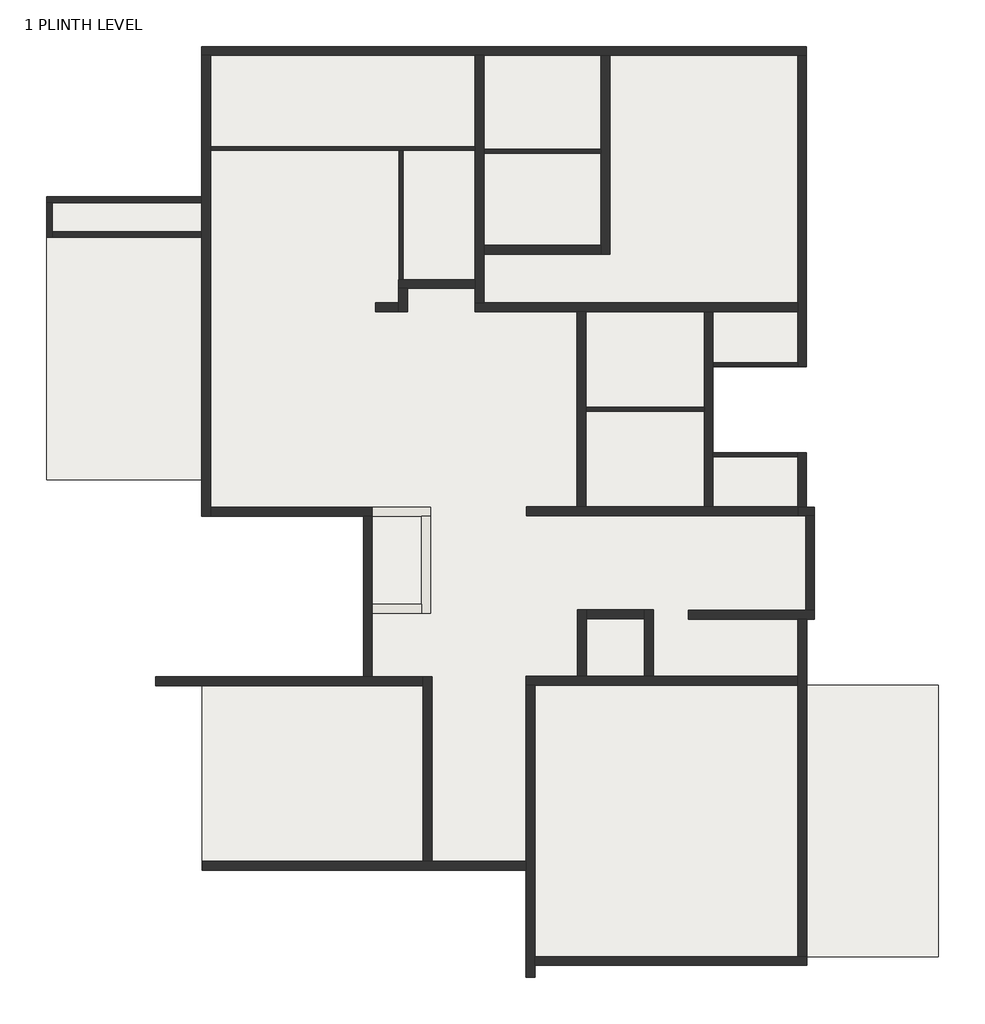
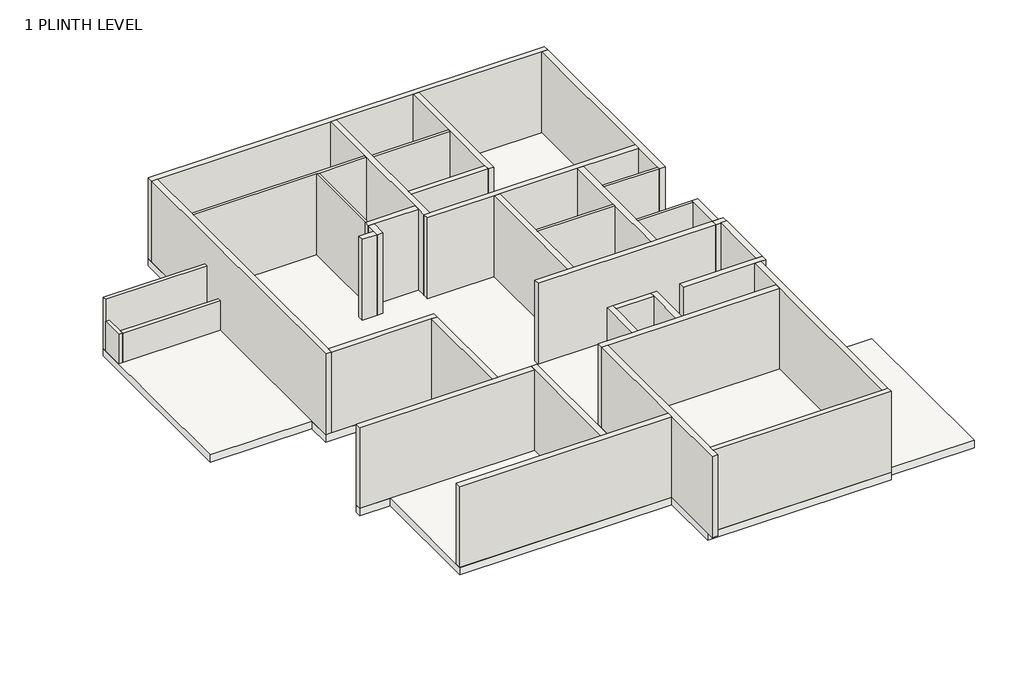
# One storey: 41 walls, 1 slab.
"""IFC4 building model written with IfcOpenShell, lengths in millimetres."""

from ifc_helpers import new_model, si_unit, frame, origin, origin_with_axes, place, context, project, spatial, polyline, outline, extrude, faceted_brep, element, save

model = new_model("IFC4")

# Units and contexts
model_context = context("Model", 3, world=origin())
ifc_project = project(units=[si_unit("LENGTHUNIT", "METRE", prefix="MILLI")], contexts=[model_context])

# Site, building, storey
site = spatial("IfcSite", under=ifc_project)
building = spatial("IfcBuilding", under=site)
storey = spatial("IfcBuildingStorey", under=building, Name="1 PLINTH LEVEL", Elevation=0.0)

# Slab
placement = place(None, origin())
element("IfcSlab", 1, ObjectType="Generic - 12\"", at=placement, inside=storey, context=model_context, shape_type="SweptSolid", body=[
    extrude(outline(polyline([(-8197.835762, 9909.3951007), (-8197.835762, 13770.1951007), (7336.8310303, 13770.1951007), (7336.8310303, 5554.9052847), (4923.8310303, 5554.9052847), (4923.8310303, 3345.1052847), (7336.8310303, 3345.1052847), (7336.8310303, 1946.9038411), (7541.4179176, 1946.9038411), (7541.4179176, -928.7689925), (7338.2179176, -928.7689925), (7338.2179176, -2623.3351307), (10716.4179176, -2623.3351307), (10716.4179176, -9591.5794723), (7338.2179176, -9591.5794723), (7338.2179176, -9820.1794723), (129.6588295, -9820.1794723), (129.6588295, -7374.0266794), (-8184.1001466, -7374.0266794), (-8184.1001466, -2640.4945725), (-9377.9001466, -2640.4945725), (-9377.9001466, -2411.8945725), (-4032.235762, -2411.8945725), (-4032.235762, 1710.0401753), (-8197.835762, 1710.0401753), (-8197.835762, 2644.9951007), (-12185.635762, 2644.9951007), (-12185.635762, 9909.3951007), (-8197.835762, 9909.3951007)])), frame((0.0, 0.0, -304.8), z_axis=(0.0, 0.0, 1.0), x_axis=(1.0, 0.0, 0.0)), (0.0, 0.0, 1.0), 304.8),
])

# Walls
element("IfcWall", 2, ObjectType="4", at=placement, inside=storey, context=model_context, shape_type="SweptSolid", body=[
    extrude(outline(polyline([(4707.9310303, 4411.490818), (1668.4271795, 4411.490818), (1668.4271795, 4513.090818), (4707.9310303, 4513.090818), (4707.9310303, 4411.490818)])), origin_with_axes(), (0.0, 0.0, 1.0), 3352.8),
])
element("IfcWall", 3, ObjectType="4", at=placement, inside=storey, context=model_context, shape_type="SweptSolid", body=[
    extrude(outline(polyline([(7108.2310303, 3243.090818), (4936.5310303, 3243.090818), (4936.5310303, 3344.690818), (7108.2310303, 3344.690818), (7108.2310303, 3243.090818)])), origin_with_axes(), (0.0, 0.0, 1.0), 3352.8),
])
element("IfcWall", 4, ObjectType="4", at=placement, inside=storey, context=model_context, shape_type="SweptSolid", body=[
    extrude(outline(polyline([(7108.8638577, 5556.2586043), (4936.5310303, 5556.2586043), (4936.5310303, 5657.8586043), (7108.8638577, 5657.8586043), (7108.8638577, 5556.2586043)])), origin_with_axes(), (0.0, 0.0, 1.0), 3352.8),
])
element("IfcWall", 5, ObjectType="4", at=placement, inside=storey, context=model_context, shape_type="SweptSolid", body=[
    extrude(outline(polyline([(2061.6821988, 11025.6870367), (-948.2178012, 11025.6870367), (-948.2178012, 11127.2870367), (2061.6821988, 11127.2870367), (2061.6821988, 11025.6870367)])), origin_with_axes(), (0.0, 0.0, 1.0), 3352.8),
])
element("IfcWall", 6, ObjectType="4", at=placement, inside=storey, context=model_context, shape_type="Brep", body=[
    faceted_brep([(-1176.8178012, 11203.4870367, 0.0), (-7969.235762, 11203.4870367, 0.0), (-7969.235762, 11203.4870367, 3352.8), (-1176.8178012, 11203.4870367, 3352.8), (-1176.8178012, 11101.8870367, 0.0), (-1176.8178012, 11101.8870367, 3352.8), (-3031.0178012, 11101.8870367, 3352.8), (-3132.6178012, 11101.8870367, 3352.8), (-7969.235762, 11101.8870367, 3352.8), (-7969.235762, 11101.8870367, 0.0), (-3132.6178012, 11101.8870367, 0.0), (-3031.0178012, 11101.8870367, 0.0)], [[[0, 1, 2, 3]], [[4, 5, 6, 7, 8, 9, 10, 11]], [[1, 0, 4, 11, 10, 9]], [[3, 2, 8, 7, 6, 5]], [[2, 1, 9, 8]], [[0, 3, 5, 4]]]),
])
element("IfcWall", 7, ObjectType="4", at=placement, inside=storey, context=model_context, shape_type="SweptSolid", body=[
    extrude(outline(polyline([(-3031.0178012, 11101.8870367), (-3031.0178012, 7787.6340845), (-3132.6178012, 7787.6340845), (-3132.6178012, 11101.8870367), (-3031.0178012, 11101.8870367)])), origin_with_axes(), (0.0, 0.0, 1.0), 3352.8),
])
element("IfcWall", 8, ObjectType="6", at=placement, inside=storey, context=model_context, shape_type="Brep", body=[
    faceted_brep([(-12185.635762, 9756.9951007, 0.0), (-12033.235762, 9756.9951007, 0.0), (-8197.835762, 9756.9951007, 0.0), (-8197.835762, 9756.9951007, 2133.6), (-12185.635762, 9756.9951007, 2133.6), (-12185.635762, 9756.9951007, 1219.2), (-12185.635762, 9909.3951007, 0.0), (-12185.635762, 9909.3951007, 2133.6), (-8197.835762, 9909.3951007, 2133.6), (-8197.835762, 9909.3951007, 0.0)], [[[0, 1, 2, 3, 4, 5]], [[6, 7, 8, 9]], [[2, 1, 0, 6, 9]], [[4, 3, 8, 7]], [[3, 2, 9, 8]], [[0, 5, 4, 7, 6]]]),
])
element("IfcWall", 9, ObjectType="6", at=placement, inside=storey, context=model_context, shape_type="Brep", body=[
    faceted_brep([(-12185.635762, 9756.9951007, 0.0), (-12185.635762, 8867.9951007, 0.0), (-12185.635762, 8867.9951007, 1219.2), (-12185.635762, 9756.9951007, 1219.2), (-12033.235762, 9756.9951007, 0.0), (-12033.235762, 9756.9951007, 1219.2), (-12033.235762, 9020.3951007, 1219.2), (-12033.235762, 8867.9951007, 1219.2), (-12033.235762, 8867.9951007, 0.0), (-12033.235762, 9020.3951007, 0.0)], [[[0, 1, 2, 3]], [[4, 5, 6, 7, 8, 9]], [[1, 0, 4, 9, 8]], [[3, 2, 7, 6, 5]], [[0, 3, 5, 4]], [[2, 1, 8, 7]]]),
])
element("IfcWall", 10, ObjectType="6", at=placement, inside=storey, context=model_context, shape_type="SweptSolid", body=[
    extrude(outline(polyline([(-8197.835762, 8867.9951007), (-12033.235762, 8867.9951007), (-12033.235762, 9020.3951007), (-8197.835762, 9020.3951007), (-8197.835762, 8867.9951007)])), origin_with_axes(), (0.0, 0.0, 1.0), 1219.2),
])
element("IfcWall", 11, ObjectType="9", at=placement, inside=storey, context=model_context, shape_type="Brep", body=[
    faceted_brep([(-8180.9354389, -7374.0266794, 0.0), (129.6588295, -7374.0266794, 0.0), (129.6588295, -7374.0266794, 3352.8), (-8180.9354389, -7374.0266794, 3352.8), (-8180.9354389, -7145.4266794, 0.0), (-8180.9354389, -7145.4266794, 3352.8), (-2516.4823872, -7145.4266794, 3352.8), (-2287.8823872, -7145.4266794, 3352.8), (129.6588295, -7145.4266794, 3352.8), (129.6588295, -7145.4266794, 0.0), (-2287.8823872, -7145.4266794, 0.0), (-2516.4823872, -7145.4266794, 0.0)], [[[0, 1, 2, 3]], [[4, 5, 6, 7, 8, 9, 10, 11]], [[1, 0, 4, 11, 10, 9]], [[3, 2, 8, 7, 6, 5]], [[0, 3, 5, 4]], [[2, 1, 9, 8]]]),
])
element("IfcWall", 12, ObjectType="9", at=placement, inside=storey, context=model_context, shape_type="Brep", body=[
    faceted_brep([(-9377.9001466, -2640.4945725, 0.0), (-2516.4823872, -2640.4945725, 0.0), (-2516.4823872, -2640.4945725, 3352.8), (-9377.9001466, -2640.4945725, 3352.8), (-9377.9001466, -2411.8945725, 0.0), (-9377.9001466, -2411.8945725, 3352.8), (-4046.9897997, -2411.8945725, 3352.8), (-3818.3897997, -2411.8945725, 3352.8), (-2516.4823872, -2411.8945725, 3352.8), (-2516.4823872, -2411.8945725, 0.0), (-3818.3897997, -2411.8945725, 0.0), (-4046.9897997, -2411.8945725, 0.0)], [[[0, 1, 2, 3]], [[4, 5, 6, 7, 8, 9, 10, 11]], [[1, 0, 4, 11, 10, 9]], [[3, 2, 8, 7, 6, 5]], [[0, 3, 5, 4]], [[2, 1, 9, 8]]]),
])
element("IfcWall", 13, ObjectType="9", at=placement, inside=storey, context=model_context, shape_type="Brep", body=[
    faceted_brep([(-2516.4823872, -2406.4280104, 0.0), (-2516.4823872, -2411.8945725, 0.0), (-2516.4823872, -2640.4945725, 0.0), (-2516.4823872, -7145.4266794, 0.0), (-2516.4823872, -7145.4266794, 3352.8), (-2516.4823872, -2640.4945725, 3352.8), (-2516.4823872, -2411.8945725, 3352.8), (-2516.4823872, -2406.4280104, 3352.8), (-2287.8823872, -2406.4280104, 0.0), (-2287.8823872, -2406.4280104, 3352.8), (-2287.8823872, -7145.4266794, 3352.8), (-2287.8823872, -7145.4266794, 0.0)], [[[0, 1, 2, 3, 4, 5, 6, 7]], [[8, 9, 10, 11]], [[3, 2, 1, 0, 8, 11]], [[7, 6, 5, 4, 10, 9]], [[0, 7, 9, 8]], [[4, 3, 11, 10]]]),
])
element("IfcWall", 14, ObjectType="9", at=placement, inside=storey, context=model_context, shape_type="Brep", body=[
    faceted_brep([(129.6588295, -2623.3351307, 0.0), (129.6588295, -7145.4266794, 0.0), (129.6588295, -7374.0266794, 0.0), (129.6588295, -10129.0351307, 0.0), (129.6588295, -10129.0351307, 3352.8), (129.6588295, -7374.0266794, 3352.8), (129.6588295, -7145.4266794, 3352.8), (129.6588295, -2623.3351307, 3352.8), (358.2588295, -2623.3351307, 0.0), (358.2588295, -2623.3351307, 3352.8), (358.2588295, -9591.5794723, 3352.8), (358.2588295, -9820.1794723, 3352.8), (358.2588295, -10129.0351307, 3352.8), (358.2588295, -10129.0351307, 0.0), (358.2588295, -9820.1794723, 0.0), (358.2588295, -9591.5794723, 0.0)], [[[0, 1, 2, 3, 4, 5, 6, 7]], [[8, 9, 10, 11, 12, 13, 14, 15]], [[3, 2, 1, 0, 8, 15, 14, 13]], [[4, 3, 13, 12]], [[7, 6, 5, 4, 12, 11, 10, 9]], [[0, 7, 9, 8]]]),
])
element("IfcWall", 15, ObjectType="9", at=placement, inside=storey, context=model_context, shape_type="Brep", body=[
    faceted_brep([(7338.2179176, -9591.5794723, 3352.8), (7338.2179176, -9591.5794723, 304.8), (7338.2179176, -9591.5794723, 0.0), (7109.6179176, -9591.5794723, 0.0), (358.2588295, -9591.5794723, 0.0), (358.2588295, -9591.5794723, 3352.8), (7109.6179176, -9591.5794723, 3352.8), (7338.2179176, -9820.1794723, 0.0), (7338.2179176, -9820.1794723, 3352.8), (358.2588295, -9820.1794723, 3352.8), (358.2588295, -9820.1794723, 0.0)], [[[0, 1, 2, 3, 4, 5, 6]], [[7, 8, 9, 10]], [[4, 3, 2, 7, 10]], [[0, 6, 5, 9, 8]], [[5, 4, 10, 9]], [[0, 8, 7, 2, 1]]]),
])
element("IfcWall", 16, ObjectType="9", at=placement, inside=storey, context=model_context, shape_type="Brep", body=[
    faceted_brep([(7338.2179176, -9591.5794723, 3352.8), (7338.2179176, -9591.5794723, 0.0), (7338.2179176, -928.7689925, 0.0), (7338.2179176, -928.7689925, 3352.8), (7109.6179176, -9591.5794723, 0.0), (7109.6179176, -9591.5794723, 3352.8), (7109.6179176, -2623.3351307, 3352.8), (7109.6179176, -2394.7351307, 3352.8), (7109.6179176, -928.7689925, 3352.8), (7109.6179176, -928.7689925, 0.0), (7109.6179176, -2394.7351307, 0.0), (7109.6179176, -2623.3351307, 0.0)], [[[0, 1, 2, 3]], [[4, 5, 6, 7, 8, 9, 10, 11]], [[2, 1, 4, 11, 10, 9]], [[0, 3, 8, 7, 6, 5]], [[3, 2, 9, 8]], [[0, 5, 4, 1]]]),
])
element("IfcWall", 17, ObjectType="9", at=placement, inside=storey, context=model_context, shape_type="Brep", body=[
    faceted_brep([(129.6588295, -2623.3351307, 0.0), (358.2588295, -2623.3351307, 0.0), (7109.6179176, -2623.3351307, 0.0), (7109.6179176, -2623.3351307, 3352.8), (358.2588295, -2623.3351307, 3352.8), (129.6588295, -2623.3351307, 3352.8), (129.6588295, -2394.7351307, 0.0), (129.6588295, -2394.7351307, 3352.8), (1455.4440373, -2394.7351307, 3352.8), (1684.0440373, -2394.7351307, 3352.8), (3168.6795302, -2394.7351307, 3352.8), (3397.2795302, -2394.7351307, 3352.8), (7109.6179176, -2394.7351307, 3352.8), (7109.6179176, -2394.7351307, 0.0), (3397.2795302, -2394.7351307, 0.0), (3168.6795302, -2394.7351307, 0.0), (1684.0440373, -2394.7351307, 0.0), (1455.4440373, -2394.7351307, 0.0)], [[[0, 1, 2, 3, 4, 5]], [[6, 7, 8, 9, 10, 11, 12, 13, 14, 15, 16, 17]], [[2, 1, 0, 6, 17, 16, 15, 14, 13]], [[5, 4, 3, 12, 11, 10, 9, 8, 7]], [[0, 5, 7, 6]], [[3, 2, 13, 12]]]),
])
element("IfcWall", 18, ObjectType="9", at=placement, inside=storey, context=model_context, shape_type="Brep", body=[
    faceted_brep([(1455.4440373, -687.9074459, 0.0), (1455.4440373, -2394.7351307, 0.0), (1455.4440373, -2394.7351307, 3352.8), (1455.4440373, -687.9074459, 3352.8), (1684.0440373, -687.9074459, 0.0), (1684.0440373, -687.9074459, 3352.8), (1684.0440373, -916.5074459, 3352.8), (1684.0440373, -2394.7351307, 3352.8), (1684.0440373, -2394.7351307, 0.0), (1684.0440373, -916.5074459, 0.0)], [[[0, 1, 2, 3]], [[4, 5, 6, 7, 8, 9]], [[1, 0, 4, 9, 8]], [[3, 2, 7, 6, 5]], [[0, 3, 5, 4]], [[2, 1, 8, 7]]]),
])
element("IfcWall", 19, ObjectType="9", at=placement, inside=storey, context=model_context, shape_type="SweptSolid", body=[
    extrude(outline(polyline([(3168.6795302, -916.5074459), (1684.0440373, -916.5074459), (1684.0440373, -687.9074459), (3168.6795302, -687.9074459), (3168.6795302, -916.5074459)])), origin_with_axes(), (0.0, 0.0, 1.0), 3352.8),
])
element("IfcWall", 20, ObjectType="9", at=placement, inside=storey, context=model_context, shape_type="Brep", body=[
    faceted_brep([(3168.6795302, -687.9074459, 0.0), (3168.6795302, -916.5074459, 0.0), (3168.6795302, -2394.7351307, 0.0), (3168.6795302, -2394.7351307, 3352.8), (3168.6795302, -916.5074459, 3352.8), (3168.6795302, -687.9074459, 3352.8), (3397.2795302, -687.9074459, 0.0), (3397.2795302, -687.9074459, 3352.8), (3397.2795302, -2394.7351307, 3352.8), (3397.2795302, -2394.7351307, 0.0)], [[[0, 1, 2, 3, 4, 5]], [[6, 7, 8, 9]], [[2, 1, 0, 6, 9]], [[5, 4, 3, 8, 7]], [[0, 5, 7, 6]], [[3, 2, 9, 8]]]),
])
element("IfcWall", 21, ObjectType="9", at=placement, inside=storey, context=model_context, shape_type="Brep", body=[
    faceted_brep([(4298.9795302, -928.7689925, 0.0), (7109.6179176, -928.7689925, 0.0), (7338.2179176, -928.7689925, 0.0), (7541.4179176, -928.7689925, 0.0), (7541.4179176, -928.7689925, 3352.8), (7338.2179176, -928.7689925, 3352.8), (7109.6179176, -928.7689925, 3352.8), (4298.9795302, -928.7689925, 3352.8), (4298.9795302, -700.1689925, 0.0), (4298.9795302, -700.1689925, 3352.8), (7312.8179176, -700.1689925, 3352.8), (7541.4179176, -700.1689925, 3352.8), (7541.4179176, -700.1689925, 0.0), (7312.8179176, -700.1689925, 0.0)], [[[0, 1, 2, 3, 4, 5, 6, 7]], [[8, 9, 10, 11, 12, 13]], [[3, 2, 1, 0, 8, 13, 12]], [[7, 6, 5, 4, 11, 10, 9]], [[0, 7, 9, 8]], [[4, 3, 12, 11]]]),
])
element("IfcWall", 22, ObjectType="9", at=placement, inside=storey, context=model_context, shape_type="Brep", body=[
    faceted_brep([(144.4271795, 1722.9180142, 0.0), (7108.2310303, 1722.9180142, 0.0), (7108.2310303, 1722.9180142, 3352.8), (144.4271795, 1722.9180142, 3352.8), (144.4271795, 1951.5180142, 0.0), (144.4271795, 1951.5180142, 3352.8), (1439.8271795, 1951.5180142, 3352.8), (1668.4271795, 1951.5180142, 3352.8), (4707.9310303, 1951.5180142, 3352.8), (4936.5310303, 1951.5180142, 3352.8), (7108.2310303, 1951.5180142, 3352.8), (7108.2310303, 1951.5180142, 0.0), (4936.5310303, 1951.5180142, 0.0), (4707.9310303, 1951.5180142, 0.0), (1668.4271795, 1951.5180142, 0.0), (1439.8271795, 1951.5180142, 0.0), (7108.2310303, 1946.9038411, 0.0), (7108.2310303, 1946.9038411, 3352.8)], [[[0, 1, 2, 3]], [[4, 5, 6, 7, 8, 9, 10, 11, 12, 13, 14, 15]], [[1, 0, 4, 15, 14, 13, 12, 11, 16]], [[3, 2, 17, 10, 9, 8, 7, 6, 5]], [[0, 3, 5, 4]], [[2, 1, 16, 11, 10, 17]]]),
])
element("IfcWall", 23, ObjectType="9", at=placement, inside=storey, context=model_context, shape_type="Brep", body=[
    faceted_brep([(7541.4179176, 1946.9038411, 3352.8), (7541.4179176, 1946.9038411, 0.0), (7336.8310303, 1946.9038411, 0.0), (7108.2310303, 1946.9038411, 0.0), (7108.2310303, 1946.9038411, 3352.8), (7336.8310303, 1946.9038411, 3352.8), (7541.4179176, 1718.3038411, 0.0), (7541.4179176, 1718.3038411, 3352.8), (7108.2310303, 1718.3038411, 3352.8), (7108.2310303, 1718.3038411, 0.0), (7108.2310303, 1722.9180142, 0.0), (7108.2310303, 1722.9180142, 3352.8)], [[[0, 1, 2, 3, 4, 5]], [[6, 7, 8, 9]], [[3, 2, 1, 6, 9, 10]], [[0, 5, 4, 11, 8, 7]], [[4, 3, 10, 9, 8, 11]], [[0, 7, 6, 1]]]),
])
element("IfcWall", 24, ObjectType="9", at=placement, inside=storey, context=model_context, shape_type="Brep", body=[
    faceted_brep([(7108.2310303, 3345.1052847, 0.0), (7108.2310303, 3344.690818, 0.0), (7108.2310303, 3243.090818, 0.0), (7108.2310303, 1951.5180142, 0.0), (7108.2310303, 1946.9038411, 0.0), (7108.2310303, 1946.9038411, 3352.8), (7108.2310303, 1951.5180142, 3352.8), (7108.2310303, 3243.090818, 3352.8), (7108.2310303, 3344.690818, 3352.8), (7108.2310303, 3345.1052847, 3352.8), (7336.8310303, 3345.1052847, 0.0), (7336.8310303, 3345.1052847, 3352.8), (7336.8310303, 1946.9038411, 3352.8), (7336.8310303, 1946.9038411, 0.0)], [[[0, 1, 2, 3, 4, 5, 6, 7, 8, 9]], [[10, 11, 12, 13]], [[4, 3, 2, 1, 0, 10, 13]], [[9, 8, 7, 6, 5, 12, 11]], [[0, 9, 11, 10]], [[5, 4, 13, 12]]]),
])
element("IfcWall", 25, ObjectType="9", at=placement, inside=storey, context=model_context, shape_type="Brep", body=[
    faceted_brep([(4936.5310303, 1951.5180142, 0.0), (4936.5310303, 3243.090818, 0.0), (4936.5310303, 3344.690818, 0.0), (4936.5310303, 5556.2586043, 0.0), (4936.5310303, 5657.8586043, 0.0), (4936.5310303, 6962.1340845, 0.0), (4936.5310303, 6962.1340845, 3352.8), (4936.5310303, 5657.8586043, 3352.8), (4936.5310303, 5556.2586043, 3352.8), (4936.5310303, 3344.690818, 3352.8), (4936.5310303, 3243.090818, 3352.8), (4936.5310303, 1951.5180142, 3352.8), (4707.9310303, 1951.5180142, 0.0), (4707.9310303, 1951.5180142, 3352.8), (4707.9310303, 4411.490818, 3352.8), (4707.9310303, 4513.090818, 3352.8), (4707.9310303, 6962.1340845, 3352.8), (4707.9310303, 6962.1340845, 0.0), (4707.9310303, 4513.090818, 0.0), (4707.9310303, 4411.490818, 0.0)], [[[0, 1, 2, 3, 4, 5, 6, 7, 8, 9, 10, 11]], [[12, 13, 14, 15, 16, 17, 18, 19]], [[5, 4, 3, 2, 1, 0, 12, 19, 18, 17]], [[11, 10, 9, 8, 7, 6, 16, 15, 14, 13]], [[0, 11, 13, 12]], [[6, 5, 17, 16]]]),
])
element("IfcWall", 26, ObjectType="9", at=placement, inside=storey, context=model_context, shape_type="Brep", body=[
    faceted_brep([(1668.4271795, 1951.5180142, 0.0), (1668.4271795, 4411.490818, 0.0), (1668.4271795, 4513.090818, 0.0), (1668.4271795, 6962.1340845, 0.0), (1668.4271795, 6962.1340845, 3352.8), (1668.4271795, 4513.090818, 3352.8), (1668.4271795, 4411.490818, 3352.8), (1668.4271795, 1951.5180142, 3352.8), (1439.8271795, 1951.5180142, 0.0), (1439.8271795, 1951.5180142, 3352.8), (1439.8271795, 6962.1340845, 3352.8), (1439.8271795, 6962.1340845, 0.0)], [[[0, 1, 2, 3, 4, 5, 6, 7]], [[8, 9, 10, 11]], [[3, 2, 1, 0, 8, 11]], [[7, 6, 5, 4, 10, 9]], [[0, 7, 9, 8]], [[4, 3, 11, 10]]]),
])
element("IfcWall", 27, ObjectType="9", at=placement, inside=storey, context=model_context, shape_type="Brep", body=[
    faceted_brep([(-8197.835762, 13541.5951007, 0.0), (-8197.835762, 9909.3951007, 0.0), (-8197.835762, 9756.9951007, 0.0), (-8197.835762, 9020.3951007, 0.0), (-8197.835762, 8867.9951007, 0.0), (-8197.835762, 1710.0401753, 0.0), (-8197.835762, 1710.0401753, 3352.8), (-8197.835762, 13541.5951007, 3352.8), (-7969.235762, 13541.5951007, 0.0), (-7969.235762, 13541.5951007, 3352.8), (-7969.235762, 11203.4870367, 3352.8), (-7969.235762, 11101.8870367, 3352.8), (-7969.235762, 1938.6401753, 3352.8), (-7969.235762, 1710.0401753, 3352.8), (-7969.235762, 1710.0401753, 0.0), (-7969.235762, 1938.6401753, 0.0), (-7969.235762, 11101.8870367, 0.0), (-7969.235762, 11203.4870367, 0.0)], [[[0, 1, 2, 3, 4, 5, 6, 7]], [[8, 9, 10, 11, 12, 13, 14, 15, 16, 17]], [[5, 4, 3, 2, 1, 0, 8, 17, 16, 15, 14]], [[7, 6, 13, 12, 11, 10, 9]], [[0, 7, 9, 8]], [[6, 5, 14, 13]]]),
])
element("IfcWall", 28, ObjectType="9", at=placement, inside=storey, context=model_context, shape_type="Brep", body=[
    faceted_brep([(-8197.835762, 13541.5951007, 0.0), (-7969.235762, 13541.5951007, 0.0), (-1176.8178012, 13541.5951007, 0.0), (-948.2178012, 13541.5951007, 0.0), (2061.6821988, 13541.5951007, 0.0), (2290.2821988, 13541.5951007, 0.0), (7108.8638577, 13541.5951007, 0.0), (7337.4638577, 13541.5951007, 0.0), (7337.4638577, 13541.5951007, 3352.8), (7108.8638577, 13541.5951007, 3352.8), (2290.2821988, 13541.5951007, 3352.8), (2061.6821988, 13541.5951007, 3352.8), (-948.2178012, 13541.5951007, 3352.8), (-1176.8178012, 13541.5951007, 3352.8), (-7969.235762, 13541.5951007, 3352.8), (-8197.835762, 13541.5951007, 3352.8), (-8197.835762, 13770.1951007, 0.0), (-8197.835762, 13770.1951007, 3352.8), (7337.4638577, 13770.1951007, 3352.8), (7337.4638577, 13770.1951007, 0.0)], [[[0, 1, 2, 3, 4, 5, 6, 7, 8, 9, 10, 11, 12, 13, 14, 15]], [[16, 17, 18, 19]], [[7, 6, 5, 4, 3, 2, 1, 0, 16, 19]], [[15, 14, 13, 12, 11, 10, 9, 8, 18, 17]], [[0, 15, 17, 16]], [[7, 19, 18, 8]]]),
])
element("IfcWall", 29, ObjectType="9", at=placement, inside=storey, context=model_context, shape_type="Brep", body=[
    faceted_brep([(7337.4638577, 5556.2586043, 0.0), (7337.4638577, 13541.5951007, 0.0), (7337.4638577, 13541.5951007, 3352.8), (7337.4638577, 5556.2586043, 3352.8), (7108.8638577, 5556.2586043, 0.0), (7108.8638577, 5556.2586043, 3352.8), (7108.8638577, 5657.8586043, 3352.8), (7108.8638577, 6962.1340845, 3352.8), (7108.8638577, 7190.7340845, 3352.8), (7108.8638577, 13541.5951007, 3352.8), (7108.8638577, 13541.5951007, 0.0), (7108.8638577, 7190.7340845, 0.0), (7108.8638577, 6962.1340845, 0.0), (7108.8638577, 5657.8586043, 0.0)], [[[0, 1, 2, 3]], [[4, 5, 6, 7, 8, 9, 10, 11, 12, 13]], [[1, 0, 4, 13, 12, 11, 10]], [[3, 2, 9, 8, 7, 6, 5]], [[0, 3, 5, 4]], [[1, 10, 9, 2]]]),
])
element("IfcWall", 30, ObjectType="9", at=placement, inside=storey, context=model_context, shape_type="Brep", body=[
    faceted_brep([(-3932.6897997, 1938.6401753, 0.0), (-7969.235762, 1938.6401753, 0.0), (-7969.235762, 1938.6401753, 3352.8), (-3818.3897997, 1938.6401753, 3352.8), (-3818.3897997, 1938.6401753, 914.4), (-3932.6897997, 1938.6401753, 914.4), (-3932.6897997, 1710.0401753, 0.0), (-3932.6897997, 1710.0401753, 914.4), (-3818.3897997, 1710.0401753, 914.4), (-3818.3897997, 1710.0401753, 3352.8), (-4046.9897997, 1710.0401753, 3352.8), (-7969.235762, 1710.0401753, 3352.8), (-7969.235762, 1710.0401753, 0.0), (-4046.9897997, 1710.0401753, 0.0)], [[[0, 1, 2, 3, 4, 5]], [[6, 7, 8, 9, 10, 11, 12, 13]], [[1, 0, 6, 13, 12]], [[3, 2, 11, 10, 9]], [[2, 1, 12, 11]], [[0, 5, 7, 6]], [[4, 8, 7, 5]], [[4, 3, 9, 8]]]),
])
element("IfcWall", 31, ObjectType="9", at=placement, inside=storey, context=model_context, shape_type="Brep", body=[
    faceted_brep([(7108.8638577, 7190.7340845, 0.0), (-948.2178012, 7190.7340845, 0.0), (-1176.8178012, 7190.7340845, 0.0), (-1176.8178012, 7190.7340845, 3352.8), (-948.2178012, 7190.7340845, 3352.8), (7108.8638577, 7190.7340845, 3352.8), (7108.8638577, 6962.1340845, 0.0), (7108.8638577, 6962.1340845, 3352.8), (4936.5310303, 6962.1340845, 3352.8), (4707.9310303, 6962.1340845, 3352.8), (1668.4271795, 6962.1340845, 3352.8), (1439.8271795, 6962.1340845, 3352.8), (-1176.8178012, 6962.1340845, 3352.8), (-1176.8178012, 6962.1340845, 0.0), (1439.8271795, 6962.1340845, 0.0), (1668.4271795, 6962.1340845, 0.0), (4707.9310303, 6962.1340845, 0.0), (4936.5310303, 6962.1340845, 0.0)], [[[0, 1, 2, 3, 4, 5]], [[6, 7, 8, 9, 10, 11, 12, 13, 14, 15, 16, 17]], [[2, 1, 0, 6, 17, 16, 15, 14, 13]], [[5, 4, 3, 12, 11, 10, 9, 8, 7]], [[0, 5, 7, 6]], [[3, 2, 13, 12]]]),
])
element("IfcWall", 32, ObjectType="9", at=placement, inside=storey, context=model_context, shape_type="Brep", body=[
    faceted_brep([(-1176.8178012, 13541.5951007, 0.0), (-1176.8178012, 11203.4870367, 0.0), (-1176.8178012, 11101.8870367, 0.0), (-1176.8178012, 7787.6340845, 0.0), (-1176.8178012, 7559.0340845, 0.0), (-1176.8178012, 7190.7340845, 0.0), (-1176.8178012, 7190.7340845, 3352.8), (-1176.8178012, 7559.0340845, 3352.8), (-1176.8178012, 7787.6340845, 3352.8), (-1176.8178012, 11101.8870367, 3352.8), (-1176.8178012, 11203.4870367, 3352.8), (-1176.8178012, 13541.5951007, 3352.8), (-948.2178012, 13541.5951007, 0.0), (-948.2178012, 13541.5951007, 3352.8), (-948.2178012, 11127.2870367, 3352.8), (-948.2178012, 11025.6870367, 3352.8), (-948.2178012, 8670.8033873, 3352.8), (-948.2178012, 8442.2033873, 3352.8), (-948.2178012, 7190.7340845, 3352.8), (-948.2178012, 7190.7340845, 0.0), (-948.2178012, 8442.2033873, 0.0), (-948.2178012, 8670.8033873, 0.0), (-948.2178012, 11025.6870367, 0.0), (-948.2178012, 11127.2870367, 0.0)], [[[0, 1, 2, 3, 4, 5, 6, 7, 8, 9, 10, 11]], [[12, 13, 14, 15, 16, 17, 18, 19, 20, 21, 22, 23]], [[5, 4, 3, 2, 1, 0, 12, 23, 22, 21, 20, 19]], [[11, 10, 9, 8, 7, 6, 18, 17, 16, 15, 14, 13]], [[0, 11, 13, 12]], [[6, 5, 19, 18]]]),
])
element("IfcWall", 33, ObjectType="9", at=placement, inside=storey, context=model_context, shape_type="Brep", body=[
    faceted_brep([(-1176.8178012, 7787.6340845, 0.0), (-3031.0178012, 7787.6340845, 0.0), (-3132.6178012, 7787.6340845, 0.0), (-3145.3178012, 7787.6340845, 0.0), (-3145.3178012, 7787.6340845, 3352.8), (-3132.6178012, 7787.6340845, 3352.8), (-3031.0178012, 7787.6340845, 3352.8), (-1176.8178012, 7787.6340845, 3352.8), (-1176.8178012, 7559.0340845, 0.0), (-1176.8178012, 7559.0340845, 3352.8), (-2916.7178012, 7559.0340845, 3352.8), (-3145.3178012, 7559.0340845, 3352.8), (-3145.3178012, 7559.0340845, 0.0), (-2916.7178012, 7559.0340845, 0.0)], [[[0, 1, 2, 3, 4, 5, 6, 7]], [[8, 9, 10, 11, 12, 13]], [[3, 2, 1, 0, 8, 13, 12]], [[7, 6, 5, 4, 11, 10, 9]], [[0, 7, 9, 8]], [[4, 3, 12, 11]]]),
])
element("IfcWall", 34, ObjectType="9", at=placement, inside=storey, context=model_context, shape_type="Brep", body=[
    faceted_brep([(-2916.7178012, 6962.1340845, 0.0), (-2916.7178012, 7559.0340845, 0.0), (-2916.7178012, 7559.0340845, 3352.8), (-2916.7178012, 6962.1340845, 3352.8), (-3145.3178012, 6962.1340845, 0.0), (-3145.3178012, 6962.1340845, 3352.8), (-3145.3178012, 7190.7340845, 3352.8), (-3145.3178012, 7559.0340845, 3352.8), (-3145.3178012, 7559.0340845, 0.0), (-3145.3178012, 7190.7340845, 0.0)], [[[0, 1, 2, 3]], [[4, 5, 6, 7, 8, 9]], [[1, 0, 4, 9, 8]], [[3, 2, 7, 6, 5]], [[0, 3, 5, 4]], [[2, 1, 8, 7]]]),
])
element("IfcWall", 35, ObjectType="9", at=placement, inside=storey, context=model_context, shape_type="SweptSolid", body=[
    extrude(outline(polyline([(-3729.5178012, 7190.7340845), (-3145.3178012, 7190.7340845), (-3145.3178012, 6962.1340845), (-3729.5178012, 6962.1340845), (-3729.5178012, 7190.7340845)])), origin_with_axes(), (0.0, 0.0, 1.0), 3352.8),
])
element("IfcWall", 36, ObjectType="9", at=placement, inside=storey, context=model_context, shape_type="Brep", body=[
    faceted_brep([(2061.6821988, 13541.5951007, 0.0), (2061.6821988, 11127.2870367, 0.0), (2061.6821988, 11025.6870367, 0.0), (2061.6821988, 8670.8033873, 0.0), (2061.6821988, 8442.2033873, 0.0), (2061.6821988, 8442.2033873, 3352.8), (2061.6821988, 8670.8033873, 3352.8), (2061.6821988, 11025.6870367, 3352.8), (2061.6821988, 11127.2870367, 3352.8), (2061.6821988, 13541.5951007, 3352.8), (2290.2821988, 13541.5951007, 0.0), (2290.2821988, 13541.5951007, 3352.8), (2290.2821988, 8442.2033873, 3352.8), (2290.2821988, 8442.2033873, 0.0)], [[[0, 1, 2, 3, 4, 5, 6, 7, 8, 9]], [[10, 11, 12, 13]], [[4, 3, 2, 1, 0, 10, 13]], [[9, 8, 7, 6, 5, 12, 11]], [[0, 9, 11, 10]], [[5, 4, 13, 12]]]),
])
element("IfcWall", 37, ObjectType="9", at=placement, inside=storey, context=model_context, shape_type="SweptSolid", body=[
    extrude(outline(polyline([(2061.6821988, 8442.2033873), (-948.2178012, 8442.2033873), (-948.2178012, 8670.8033873), (2061.6821988, 8670.8033873), (2061.6821988, 8442.2033873)])), origin_with_axes(), (0.0, 0.0, 1.0), 3352.8),
])
element("IfcWall", 38, ObjectType="9", at=placement, inside=storey, context=model_context, shape_type="SweptSolid", body=[
    extrude(outline(polyline([(7541.4179176, 1722.9180142), (7541.4179176, -700.1689925), (7312.8179176, -700.1689925), (7312.8179176, 1722.9180142), (7541.4179176, 1722.9180142)])), origin_with_axes(), (0.0, 0.0, 1.0), 3352.8),
])
element("IfcWall", 39, ObjectType="9", at=placement, inside=storey, context=model_context, shape_type="Brep", body=[
    faceted_brep([(-3932.6897997, 1710.0401753, 0.0), (-3818.3897997, 1710.0401753, 0.0), (-2548.3897997, 1710.0401753, 0.0), (-2319.7897997, 1710.0401753, 0.0), (-2319.7897997, 1710.0401753, 914.4), (-2548.3897997, 1710.0401753, 914.4), (-3818.3897997, 1710.0401753, 914.4), (-3932.6897997, 1710.0401753, 914.4), (-3932.6897997, 1938.6401753, 0.0), (-3932.6897997, 1938.6401753, 914.4), (-3818.3897997, 1938.6401753, 914.4), (-2319.7897997, 1938.6401753, 914.4), (-2319.7897997, 1938.6401753, 0.0)], [[[0, 1, 2, 3, 4, 5, 6, 7]], [[8, 9, 10, 11, 12]], [[3, 2, 1, 0, 8, 12]], [[7, 6, 5, 4, 11, 10, 9]], [[0, 7, 9, 8]], [[4, 3, 12, 11]]]),
])
element("IfcWall", 40, ObjectType="9", at=placement, inside=storey, context=model_context, shape_type="Brep", body=[
    faceted_brep([(-2548.3897997, 1710.0401753, 0.0), (-2548.3897997, -550.5598247, 0.0), (-2548.3897997, -779.1598247, 0.0), (-2548.3897997, -779.1598247, 914.4), (-2548.3897997, -550.5598247, 914.4), (-2548.3897997, 1710.0401753, 914.4), (-2319.7897997, 1710.0401753, 0.0), (-2319.7897997, 1710.0401753, 914.4), (-2319.7897997, -779.1598247, 914.4), (-2319.7897997, -779.1598247, 0.0)], [[[0, 1, 2, 3, 4, 5]], [[6, 7, 8, 9]], [[2, 1, 0, 6, 9]], [[5, 4, 3, 8, 7]], [[0, 5, 7, 6]], [[3, 2, 9, 8]]]),
])
element("IfcWall", 41, ObjectType="9", at=placement, inside=storey, context=model_context, shape_type="SweptSolid", body=[
    extrude(outline(polyline([(-3818.3897997, -550.5598247), (-2548.3897997, -550.5598247), (-2548.3897997, -779.1598247), (-3818.3897997, -779.1598247), (-3818.3897997, -550.5598247)])), origin_with_axes(), (0.0, 0.0, 1.0), 914.4),
])
element("IfcWall", 42, ObjectType="9", at=placement, inside=storey, context=model_context, shape_type="Brep", body=[
    faceted_brep([(-4046.9897997, 1710.0401753, 3352.8), (-4046.9897997, 1710.0401753, 0.0), (-4046.9897997, -2411.8945725, 0.0), (-4046.9897997, -2411.8945725, 3352.8), (-3818.3897997, 1710.0401753, 0.0), (-3818.3897997, 1710.0401753, 914.4), (-3818.3897997, 1710.0401753, 3352.8), (-3818.3897997, -2411.8945725, 3352.8), (-3818.3897997, -2411.8945725, 0.0), (-3818.3897997, -779.1598247, 0.0), (-3818.3897997, -550.5598247, 0.0), (-3932.6897997, 1710.0401753, 0.0)], [[[0, 1, 2, 3]], [[4, 5, 6, 7, 8, 9, 10]], [[2, 1, 11, 4, 10, 9, 8]], [[0, 3, 7, 6]], [[0, 6, 5, 4, 11, 1]], [[3, 2, 8, 7]]]),
])

save(model, "model.ifc")

# Revit data of these elements
# Type "Generic - 12\""
#   Assembly Code = "B1010"
#   Function = 0
#   Layers, outside or top first: 1' - 0" no material (function 1)
# Type "4"
#   Assembly Code = "B2010"
#   Layers, outside or top first: 0' - 4" no material (function 1)
# Type "6"
#   Assembly Code = "B2010"
#   Layers, outside or top first: 0' - 6" no material (function 1)
# Type "9"
#   Assembly Code = "B2010"
#   Layers, outside or top first: 0' - 9" no material (function 1)
# Element 1 (IfcSlab, "Generic - 12\"")
#   built-in parameter 1001955 = -1.5708 (stored number, unit not read)
#   Height Offset From Level = 0' - 0"
#   Phase Created = New Construction
#   Materials on its faces: "Default Floor"
# Elements 2, 3, 4, 5, 6, 7 (IfcWall, "4")
#   Top Offset = 0' - 0"
#   Base Offset = 0' - 0"
#   wall height = 11' - 0"
#   Phase Created = New Construction
#   Base Constraint = 1 PLINTH LEVEL
#   Top Constraint = 2 FIRST FLOOR BASE
#   Materials on its faces: "Default Wall"
# Element 8 (IfcWall, "6")
#   Top Offset = 0' - 0"
#   Base Offset = 0' - 0"
#   Unconnected Height = 7' - 0"
#   wall height = 7' - 0"
#   Phase Created = New Construction
#   Base Constraint = 1 PLINTH LEVEL
#   Materials on its faces: "Default Wall"
# Elements 9, 10 (IfcWall, "6")
#   Top Offset = 0' - 0"
#   Base Offset = 0' - 0"
#   Unconnected Height = 4' - 0"
#   wall height = 4' - 0"
#   Phase Created = New Construction
#   Base Constraint = 1 PLINTH LEVEL
#   Materials on its faces: "Default Wall"
# Elements 11, 12, 13, 14, 15, 16, 17, 18, 19, 20, 21, 22, 23, 24, 25, 26, 27, 28, 29, 30, 31, 32, 33, 34, 35, 36, 37, 38, 42 (IfcWall, "9")
#   Top Offset = 0' - 0"
#   Base Offset = 0' - 0"
#   wall height = 11' - 0"
#   Phase Created = New Construction
#   Base Constraint = 1 PLINTH LEVEL
#   Top Constraint = 2 FIRST FLOOR BASE
#   Materials on its faces: "Default Wall"
# Elements 39, 40, 41 (IfcWall, "9")
#   Top Offset = 0' - 0"
#   Base Offset = 0' - 0"
#   Unconnected Height = 3' - 0"
#   wall height = 3' - 0"
#   Phase Created = New Construction
#   Base Constraint = 1 PLINTH LEVEL
#   Materials on its faces: "Default Wall"
# Materials
#   "Default Floor": colour RGB 128 128 128, transparency 0, Cost = 0
#   "Default Wall": colour RGB 128 128 128, transparency 0, Cost = 0
